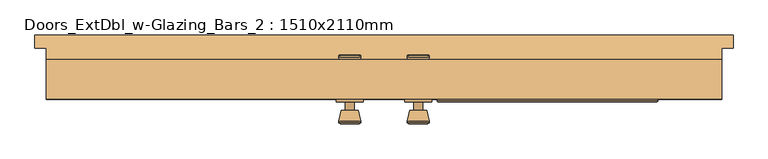
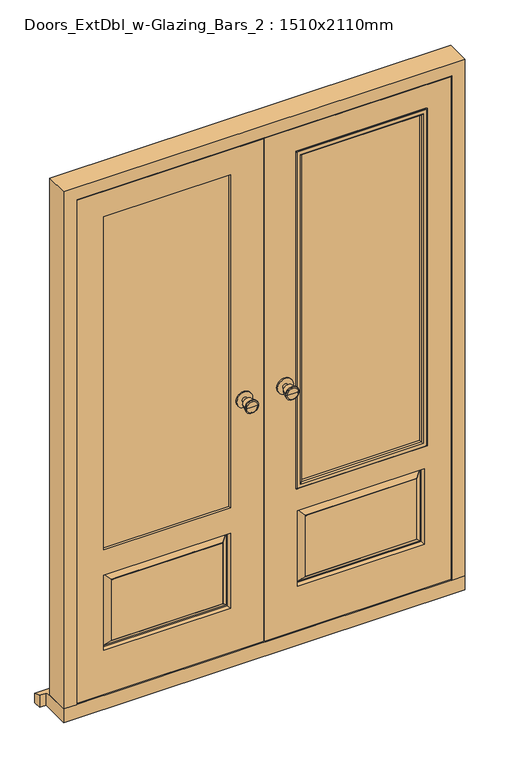
"""IFC4 building model written with IfcOpenShell, lengths in millimetres: door geometry, Doors_ExtDbl_w-Glazing_Bars_2 : 1510x2110mm."""

from ifc_helpers import new_model, si_unit, point, frame, frame_2d, origin, place, context, project, spatial, polyline, circle_curve, ellipse_curve, trimmed, segment, composite_curve, outline, extrude, faceted_brep, source, transform, mapped, element, save
from ifc_brep_helpers import plane_surface, cylinder_surface, revolved_surface, advanced_brep


def doors_extdbl_w_glazing_bars_2_1510x2110mm_e5cd3545(model_context):
    return source(origin(), model_context, "Body", "SolidModel", [
        advanced_brep(
        [(76.5, -18.4, 1050.0), (86.5, -18.4, 1050.0), (66.5, -18.4, 1050.0), (96.9758676, -67.4, 1050.0), (76.5, -67.4, 1050.0), (56.0241324, -67.4, 1050.0), (101.5, -65.5721319, 1050.0), (51.5, -65.5721319, 1050.0), (101.5, -62.1084537, 1050.0), (51.5, -62.1084537, 1050.0), (95.136236, -37.4, 1050.0), (57.863764, -37.4, 1050.0), (86.5, -37.4, 1050.0), (66.5, -37.4, 1050.0)],
        [
            (0, 1),
            (1, 2, circle_curve(frame((76.5, -18.4, 1050.0), z_axis=(0.0, 1.0, 0.0), x_axis=(-1.0, 0.0, 0.0)), 10.0)),
            (2, 0),
            (2, 1, circle_curve(frame((76.5, -18.4, 1050.0), z_axis=(0.0, 1.0, 0.0), x_axis=(-1.0, 0.0, 0.0)), 10.0)),
            (3, 4),
            (4, 5),
            (5, 3, circle_curve(frame((76.5, -67.4, 1050.0), z_axis=(0.0, -1.0, 0.0), x_axis=(-1.0, 0.0, 0.0)), 20.4758676)),
            (3, 5, circle_curve(frame((76.5, -67.4, 1050.0), z_axis=(0.0, -1.0, 0.0), x_axis=(-1.0, 0.0, 0.0)), 20.4758676)),
            (6, 3),
            (5, 7),
            (7, 6, circle_curve(frame((76.5, -65.5721319, 1050.0), z_axis=(0.0, -1.0, 0.0), x_axis=(-1.0, 0.0, 0.0)), 25.0)),
            (6, 7, circle_curve(frame((76.5, -65.5721319, 1050.0), z_axis=(0.0, -1.0, 0.0), x_axis=(-1.0, 0.0, 0.0)), 25.0)),
            (8, 6),
            (7, 9),
            (9, 8, circle_curve(frame((76.5, -62.1084537, 1050.0), z_axis=(0.0, -1.0, 0.0), x_axis=(-1.0, 0.0, 0.0)), 25.0)),
            (8, 9, circle_curve(frame((76.5, -62.1084537, 1050.0), z_axis=(0.0, -1.0, 0.0), x_axis=(-1.0, 0.0, 0.0)), 25.0)),
            (10, 8),
            (9, 11),
            (11, 10, circle_curve(frame((76.5, -37.4, 1050.0), z_axis=(0.0, -1.0, 0.0), x_axis=(-1.0, 0.0, 0.0)), 18.636236)),
            (10, 11, circle_curve(frame((76.5, -37.4, 1050.0), z_axis=(0.0, -1.0, 0.0), x_axis=(-1.0, 0.0, 0.0)), 18.636236)),
            (12, 10),
            (11, 13),
            (13, 12, circle_curve(frame((76.5, -37.4, 1050.0), z_axis=(0.0, -1.0, 0.0), x_axis=(-1.0, 0.0, 0.0)), 10.0)),
            (12, 13, circle_curve(frame((76.5, -37.4, 1050.0), z_axis=(0.0, -1.0, 0.0), x_axis=(-1.0, 0.0, 0.0)), 10.0)),
            (1, 12),
            (13, 2),
        ],
        [
            plane_surface(frame((76.5, -18.4, 1050.0), z_axis=(0.0, 1.0, 0.0), x_axis=(-1.0, 0.0, 0.0))),
            plane_surface(frame((76.5, -67.4, 1050.0), z_axis=(0.0, -1.0, 0.0), x_axis=(-1.0, 0.0, 0.0))),
            revolved_surface(polyline([(56.0241324, -67.4, 1050.0), (51.5, -65.5721319, 1050.0)]), (76.5, -18.4, 1050.0), (0.0, 1.0, 0.0)),
            cylinder_surface(frame((76.5, -18.4, 1050.0), z_axis=(0.0, 1.0, 0.0), x_axis=(-1.0, 0.0, 0.0)), 25.0),
            revolved_surface(polyline([(51.5, -62.1084537, 1050.0), (57.863764, -37.4, 1050.0)]), (76.5, -18.4, 1050.0), (0.0, 1.0, 0.0)),
            plane_surface(frame((76.5, -37.4, 1050.0), z_axis=(0.0, 1.0, 0.0), x_axis=(-1.0, 0.0, 0.0))),
            cylinder_surface(frame((76.5, -18.4, 1050.0), z_axis=(0.0, 1.0, 0.0), x_axis=(-1.0, 0.0, 0.0)), 10.0),
        ],
        [
            (0, [[1, 2, 3]]),
            (0, [[-3, 4, -1]]),
            (1, [[5, 6, 7]]),
            (1, [[-6, -5, 8]]),
            (2, [[9, -7, 10, 11]]),
            (2, [[-10, -8, -9, 12]]),
            (3, [[13, -11, 14, 15]]),
            (3, [[-14, -12, -13, 16]]),
            (4, [[17, -15, 18, 19]]),
            (4, [[-18, -16, -17, 20]]),
            (5, [[21, -19, 22, 23]]),
            (5, [[-22, -20, -21, 24]]),
            (6, [[25, -23, 26, -2]]),
            (6, [[-26, -24, -25, -4]]),
        ],
    ),
        extrude(outline(composite_curve([segment(trimmed(circle_curve(frame_2d((1050.0, 76.5)), 30.0), [point((1050.0, 46.5))], [point((1050.0, 106.5))], False, "CARTESIAN"), True, "CONTINUOUS"), segment(trimmed(circle_curve(frame_2d((1050.0, 76.5)), 30.0), [point((1050.0, 106.5))], [point((1050.0, 46.5))], False, "CARTESIAN"), True, "CONTINUOUS")], self_intersect=False)), frame((0.0, -18.4, 0.0), z_axis=(0.0, 1.0, 0.0), x_axis=(0.0, 0.0, 1.0)), (0.0, 0.0, 1.0), 6.0),
        advanced_brep(
        [(76.5, 37.6, 1050.0), (66.5, 37.6, 1050.0), (86.5, 37.6, 1050.0), (96.9758676, 86.6, 1050.0), (56.0241324, 86.6, 1050.0), (76.5, 86.6, 1050.0), (101.5, 84.7721319, 1050.0), (51.5, 84.7721319, 1050.0), (101.5, 81.3084537, 1050.0), (51.5, 81.3084537, 1050.0), (95.136236, 56.6, 1050.0), (57.863764, 56.6, 1050.0), (86.5, 56.6, 1050.0), (66.5, 56.6, 1050.0)],
        [
            (0, 1),
            (1, 2, circle_curve(frame((76.5, 37.6, 1050.0), z_axis=(0.0, -1.0, 0.0), x_axis=(-1.0, 0.0, 0.0)), 10.0)),
            (2, 0),
            (2, 1, circle_curve(frame((76.5, 37.6, 1050.0), z_axis=(0.0, -1.0, 0.0), x_axis=(-1.0, 0.0, 0.0)), 10.0)),
            (3, 4, circle_curve(frame((76.5, 86.6, 1050.0), z_axis=(0.0, 1.0, 0.0), x_axis=(-1.0, 0.0, 0.0)), 20.4758676)),
            (4, 5),
            (5, 3),
            (4, 3, circle_curve(frame((76.5, 86.6, 1050.0), z_axis=(0.0, 1.0, 0.0), x_axis=(-1.0, 0.0, 0.0)), 20.4758676)),
            (6, 7, circle_curve(frame((76.5, 84.7721319, 1050.0), z_axis=(0.0, 1.0, 0.0), x_axis=(-1.0, 0.0, 0.0)), 25.0)),
            (7, 4),
            (3, 6),
            (7, 6, circle_curve(frame((76.5, 84.7721319, 1050.0), z_axis=(0.0, 1.0, 0.0), x_axis=(-1.0, 0.0, 0.0)), 25.0)),
            (8, 9, circle_curve(frame((76.5, 81.3084537, 1050.0), z_axis=(0.0, 1.0, 0.0), x_axis=(-1.0, 0.0, 0.0)), 25.0)),
            (9, 7),
            (6, 8),
            (9, 8, circle_curve(frame((76.5, 81.3084537, 1050.0), z_axis=(0.0, 1.0, 0.0), x_axis=(-1.0, 0.0, 0.0)), 25.0)),
            (10, 11, circle_curve(frame((76.5, 56.6, 1050.0), z_axis=(0.0, 1.0, 0.0), x_axis=(-1.0, 0.0, 0.0)), 18.636236)),
            (11, 9),
            (8, 10),
            (11, 10, circle_curve(frame((76.5, 56.6, 1050.0), z_axis=(0.0, 1.0, 0.0), x_axis=(-1.0, 0.0, 0.0)), 18.636236)),
            (12, 13, circle_curve(frame((76.5, 56.6, 1050.0), z_axis=(0.0, 1.0, 0.0), x_axis=(-1.0, 0.0, 0.0)), 10.0)),
            (13, 11),
            (10, 12),
            (13, 12, circle_curve(frame((76.5, 56.6, 1050.0), z_axis=(0.0, 1.0, 0.0), x_axis=(-1.0, 0.0, 0.0)), 10.0)),
            (1, 13),
            (12, 2),
        ],
        [
            plane_surface(frame((76.5, 37.6, 1050.0), z_axis=(0.0, -1.0, 0.0), x_axis=(-1.0, 0.0, 0.0))),
            plane_surface(frame((76.5, 86.6, 1050.0), z_axis=(0.0, 1.0, 0.0), x_axis=(-1.0, 0.0, 0.0))),
            revolved_surface(polyline([(56.0241324, 86.6, 1050.0), (51.5, 84.7721319, 1050.0)]), (76.5, 37.6, 1050.0), (0.0, -1.0, 0.0)),
            cylinder_surface(frame((76.5, 37.6, 1050.0), z_axis=(0.0, -1.0, 0.0), x_axis=(-1.0, 0.0, 0.0)), 25.0),
            revolved_surface(polyline([(51.5, 81.3084537, 1050.0), (57.863764, 56.6, 1050.0)]), (76.5, 37.6, 1050.0), (0.0, -1.0, 0.0)),
            plane_surface(frame((76.5, 56.6, 1050.0), z_axis=(0.0, -1.0, 0.0), x_axis=(-1.0, 0.0, 0.0))),
            cylinder_surface(frame((76.5, 37.6, 1050.0), z_axis=(0.0, -1.0, 0.0), x_axis=(-1.0, 0.0, 0.0)), 10.0),
        ],
        [
            (0, [[1, 2, 3]]),
            (0, [[-3, 4, -1]]),
            (1, [[5, 6, 7]]),
            (1, [[8, -7, -6]]),
            (2, [[9, 10, -5, 11]]),
            (2, [[12, -11, -8, -10]]),
            (3, [[13, 14, -9, 15]]),
            (3, [[16, -15, -12, -14]]),
            (4, [[17, 18, -13, 19]]),
            (4, [[20, -19, -16, -18]]),
            (5, [[21, 22, -17, 23]]),
            (5, [[24, -23, -20, -22]]),
            (6, [[-2, 25, -21, 26]]),
            (6, [[-4, -26, -24, -25]]),
        ],
    ),
        extrude(outline(composite_curve([segment(trimmed(circle_curve(frame_2d((1050.0, 76.5)), 30.0), [point((1050.0, 46.5))], [point((1050.0, 106.5))], False, "CARTESIAN"), True, "CONTINUOUS"), segment(trimmed(circle_curve(frame_2d((1050.0, 76.5)), 30.0), [point((1050.0, 106.5))], [point((1050.0, 46.5))], False, "CARTESIAN"), True, "CONTINUOUS")], self_intersect=False)), frame((0.0, 31.6, 0.0), z_axis=(0.0, 1.0, 0.0), x_axis=(0.0, 0.0, 1.0)), (0.0, 0.0, 1.0), 6.0),
        advanced_brep(
        [(-76.5, -18.4, 1050.0), (-66.5, -18.4, 1050.0), (-86.5, -18.4, 1050.0), (-56.0241324, -67.4, 1050.0), (-76.5, -67.4, 1050.0), (-96.9758676, -67.4, 1050.0), (-51.5, -65.5721319, 1050.0), (-101.5, -65.5721319, 1050.0), (-51.5, -62.1084537, 1050.0), (-101.5, -62.1084537, 1050.0), (-57.863764, -37.4, 1050.0), (-95.136236, -37.4, 1050.0), (-66.5, -37.4, 1050.0), (-86.5, -37.4, 1050.0)],
        [
            (0, 1),
            (1, 2, circle_curve(frame((-76.5, -18.4, 1050.0), z_axis=(0.0, 1.0, 0.0), x_axis=(-1.0, 0.0, 0.0)), 10.0)),
            (2, 0),
            (2, 1, circle_curve(frame((-76.5, -18.4, 1050.0), z_axis=(0.0, 1.0, 0.0), x_axis=(-1.0, 0.0, 0.0)), 10.0)),
            (3, 4),
            (4, 5),
            (5, 3, circle_curve(frame((-76.5, -67.4, 1050.0), z_axis=(0.0, -1.0, 0.0), x_axis=(-1.0, 0.0, 0.0)), 20.4758676)),
            (3, 5, circle_curve(frame((-76.5, -67.4, 1050.0), z_axis=(0.0, -1.0, 0.0), x_axis=(-1.0, 0.0, 0.0)), 20.4758676)),
            (6, 3),
            (5, 7),
            (7, 6, circle_curve(frame((-76.5, -65.5721319, 1050.0), z_axis=(0.0, -1.0, 0.0), x_axis=(-1.0, 0.0, 0.0)), 25.0)),
            (6, 7, circle_curve(frame((-76.5, -65.5721319, 1050.0), z_axis=(0.0, -1.0, 0.0), x_axis=(-1.0, 0.0, 0.0)), 25.0)),
            (8, 6),
            (7, 9),
            (9, 8, circle_curve(frame((-76.5, -62.1084537, 1050.0), z_axis=(0.0, -1.0, 0.0), x_axis=(-1.0, 0.0, 0.0)), 25.0)),
            (8, 9, circle_curve(frame((-76.5, -62.1084537, 1050.0), z_axis=(0.0, -1.0, 0.0), x_axis=(-1.0, 0.0, 0.0)), 25.0)),
            (10, 8),
            (9, 11),
            (11, 10, circle_curve(frame((-76.5, -37.4, 1050.0), z_axis=(0.0, -1.0, 0.0), x_axis=(-1.0, 0.0, 0.0)), 18.636236)),
            (10, 11, circle_curve(frame((-76.5, -37.4, 1050.0), z_axis=(0.0, -1.0, 0.0), x_axis=(-1.0, 0.0, 0.0)), 18.636236)),
            (12, 10),
            (11, 13),
            (13, 12, circle_curve(frame((-76.5, -37.4, 1050.0), z_axis=(0.0, -1.0, 0.0), x_axis=(-1.0, 0.0, 0.0)), 10.0)),
            (12, 13, circle_curve(frame((-76.5, -37.4, 1050.0), z_axis=(0.0, -1.0, 0.0), x_axis=(-1.0, 0.0, 0.0)), 10.0)),
            (1, 12),
            (13, 2),
        ],
        [
            plane_surface(frame((-76.5, -18.4, 1050.0), z_axis=(0.0, 1.0, 0.0), x_axis=(-1.0, 0.0, 0.0))),
            plane_surface(frame((-76.5, -67.4, 1050.0), z_axis=(0.0, -1.0, 0.0), x_axis=(-1.0, 0.0, 0.0))),
            revolved_surface(polyline([(-96.9758676, -67.4, 1050.0), (-101.5, -65.5721319, 1050.0)]), (-76.5, -18.4, 1050.0), (0.0, 1.0, 0.0)),
            cylinder_surface(frame((-76.5, -18.4, 1050.0), z_axis=(0.0, 1.0, 0.0), x_axis=(-1.0, 0.0, 0.0)), 25.0),
            revolved_surface(polyline([(-101.5, -62.1084537, 1050.0), (-95.136236, -37.4, 1050.0)]), (-76.5, -18.4, 1050.0), (0.0, 1.0, 0.0)),
            plane_surface(frame((-76.5, -37.4, 1050.0), z_axis=(0.0, 1.0, 0.0), x_axis=(-1.0, 0.0, 0.0))),
            cylinder_surface(frame((-76.5, -18.4, 1050.0), z_axis=(0.0, 1.0, 0.0), x_axis=(-1.0, 0.0, 0.0)), 10.0),
        ],
        [
            (0, [[1, 2, 3]]),
            (0, [[-3, 4, -1]]),
            (1, [[5, 6, 7]]),
            (1, [[-6, -5, 8]]),
            (2, [[9, -7, 10, 11]]),
            (2, [[-10, -8, -9, 12]]),
            (3, [[13, -11, 14, 15]]),
            (3, [[-14, -12, -13, 16]]),
            (4, [[17, -15, 18, 19]]),
            (4, [[-18, -16, -17, 20]]),
            (5, [[21, -19, 22, 23]]),
            (5, [[-22, -20, -21, 24]]),
            (6, [[25, -23, 26, -2]]),
            (6, [[-26, -24, -25, -4]]),
        ],
    ),
        extrude(outline(composite_curve([segment(trimmed(circle_curve(frame_2d((1050.0, -76.5)), 30.0), [point((1050.0, -106.5))], [point((1050.0, -46.5))], False, "CARTESIAN"), True, "CONTINUOUS"), segment(trimmed(circle_curve(frame_2d((1050.0, -76.5)), 30.0), [point((1050.0, -46.5))], [point((1050.0, -106.5))], False, "CARTESIAN"), True, "CONTINUOUS")], self_intersect=False)), frame((0.0, -18.4, 0.0), z_axis=(0.0, 1.0, 0.0), x_axis=(0.0, 0.0, 1.0)), (0.0, 0.0, 1.0), 6.0),
        advanced_brep(
        [(-76.5, 37.6, 1050.0), (-86.5, 37.6, 1050.0), (-66.5, 37.6, 1050.0), (-56.0241324, 86.6, 1050.0), (-96.9758676, 86.6, 1050.0), (-76.5, 86.6, 1050.0), (-51.5, 84.7721319, 1050.0), (-101.5, 84.7721319, 1050.0), (-51.5, 81.3084537, 1050.0), (-101.5, 81.3084537, 1050.0), (-57.863764, 56.6, 1050.0), (-95.136236, 56.6, 1050.0), (-66.5, 56.6, 1050.0), (-86.5, 56.6, 1050.0)],
        [
            (0, 1),
            (1, 2, circle_curve(frame((-76.5, 37.6, 1050.0), z_axis=(0.0, -1.0, 0.0), x_axis=(-1.0, 0.0, 0.0)), 10.0)),
            (2, 0),
            (2, 1, circle_curve(frame((-76.5, 37.6, 1050.0), z_axis=(0.0, -1.0, 0.0), x_axis=(-1.0, 0.0, 0.0)), 10.0)),
            (3, 4, circle_curve(frame((-76.5, 86.6, 1050.0), z_axis=(0.0, 1.0, 0.0), x_axis=(-1.0, 0.0, 0.0)), 20.4758676)),
            (4, 5),
            (5, 3),
            (4, 3, circle_curve(frame((-76.5, 86.6, 1050.0), z_axis=(0.0, 1.0, 0.0), x_axis=(-1.0, 0.0, 0.0)), 20.4758676)),
            (6, 7, circle_curve(frame((-76.5, 84.7721319, 1050.0), z_axis=(0.0, 1.0, 0.0), x_axis=(-1.0, 0.0, 0.0)), 25.0)),
            (7, 4),
            (3, 6),
            (7, 6, circle_curve(frame((-76.5, 84.7721319, 1050.0), z_axis=(0.0, 1.0, 0.0), x_axis=(-1.0, 0.0, 0.0)), 25.0)),
            (8, 9, circle_curve(frame((-76.5, 81.3084537, 1050.0), z_axis=(0.0, 1.0, 0.0), x_axis=(-1.0, 0.0, 0.0)), 25.0)),
            (9, 7),
            (6, 8),
            (9, 8, circle_curve(frame((-76.5, 81.3084537, 1050.0), z_axis=(0.0, 1.0, 0.0), x_axis=(-1.0, 0.0, 0.0)), 25.0)),
            (10, 11, circle_curve(frame((-76.5, 56.6, 1050.0), z_axis=(0.0, 1.0, 0.0), x_axis=(-1.0, 0.0, 0.0)), 18.636236)),
            (11, 9),
            (8, 10),
            (11, 10, circle_curve(frame((-76.5, 56.6, 1050.0), z_axis=(0.0, 1.0, 0.0), x_axis=(-1.0, 0.0, 0.0)), 18.636236)),
            (12, 13, circle_curve(frame((-76.5, 56.6, 1050.0), z_axis=(0.0, 1.0, 0.0), x_axis=(-1.0, 0.0, 0.0)), 10.0)),
            (13, 11),
            (10, 12),
            (13, 12, circle_curve(frame((-76.5, 56.6, 1050.0), z_axis=(0.0, 1.0, 0.0), x_axis=(-1.0, 0.0, 0.0)), 10.0)),
            (1, 13),
            (12, 2),
        ],
        [
            plane_surface(frame((-76.5, 37.6, 1050.0), z_axis=(0.0, -1.0, 0.0), x_axis=(-1.0, 0.0, 0.0))),
            plane_surface(frame((-76.5, 86.6, 1050.0), z_axis=(0.0, 1.0, 0.0), x_axis=(-1.0, 0.0, 0.0))),
            revolved_surface(polyline([(-96.9758676, 86.6, 1050.0), (-101.5, 84.7721319, 1050.0)]), (-76.5, 37.6, 1050.0), (0.0, -1.0, 0.0)),
            cylinder_surface(frame((-76.5, 37.6, 1050.0), z_axis=(0.0, -1.0, 0.0), x_axis=(-1.0, 0.0, 0.0)), 25.0),
            revolved_surface(polyline([(-101.5, 81.3084537, 1050.0), (-95.136236, 56.6, 1050.0)]), (-76.5, 37.6, 1050.0), (0.0, -1.0, 0.0)),
            plane_surface(frame((-76.5, 56.6, 1050.0), z_axis=(0.0, -1.0, 0.0), x_axis=(-1.0, 0.0, 0.0))),
            cylinder_surface(frame((-76.5, 37.6, 1050.0), z_axis=(0.0, -1.0, 0.0), x_axis=(-1.0, 0.0, 0.0)), 10.0),
        ],
        [
            (0, [[1, 2, 3]]),
            (0, [[-3, 4, -1]]),
            (1, [[5, 6, 7]]),
            (1, [[8, -7, -6]]),
            (2, [[9, 10, -5, 11]]),
            (2, [[12, -11, -8, -10]]),
            (3, [[13, 14, -9, 15]]),
            (3, [[16, -15, -12, -14]]),
            (4, [[17, 18, -13, 19]]),
            (4, [[20, -19, -16, -18]]),
            (5, [[21, 22, -17, 23]]),
            (5, [[24, -23, -20, -22]]),
            (6, [[-2, 25, -21, 26]]),
            (6, [[-4, -26, -24, -25]]),
        ],
    ),
        extrude(outline(composite_curve([segment(trimmed(circle_curve(frame_2d((1050.0, -76.5)), 30.0), [point((1050.0, -106.5))], [point((1050.0, -46.5))], False, "CARTESIAN"), True, "CONTINUOUS"), segment(trimmed(circle_curve(frame_2d((1050.0, -76.5)), 30.0), [point((1050.0, -46.5))], [point((1050.0, -106.5))], False, "CARTESIAN"), True, "CONTINUOUS")], self_intersect=False)), frame((0.0, 31.6, 0.0), z_axis=(0.0, 1.0, 0.0), x_axis=(0.0, 0.0, 1.0)), (0.0, 0.0, 1.0), 6.0),
        faceted_brep([(684.5, 76.6, 54.5), (755.0, 76.6, 54.5), (755.0, -12.4, 54.5), (706.5, -12.4, 54.5), (706.5, 34.6, 54.5), (684.5, 34.6, 54.5), (684.5, 76.6, 2039.5), (-684.5, 76.6, 2039.5), (-684.5, 76.6, 54.5), (-755.0, 76.6, 54.5), (-755.0, 76.6, 2110.0), (755.0, 76.6, 2110.0), (755.0, -12.4, 2110.0), (-755.0, -12.4, 2110.0), (-755.0, -12.4, 54.5), (-706.5, -12.4, 54.5), (-706.5, -12.4, 2061.5), (706.5, -12.4, 2061.5), (706.5, 34.6, 2061.5), (-706.5, 34.6, 2061.5), (-706.5, 34.6, 54.5), (-684.5, 34.6, 54.5), (-684.5, 34.6, 2039.5), (684.5, 34.6, 2039.5)], [[[0, 1, 2, 3, 4, 5]], [[1, 0, 6, 7, 8, 9, 10, 11]], [[2, 1, 11, 12]], [[3, 2, 12, 13, 14, 15, 16, 17]], [[4, 3, 17, 18]], [[5, 4, 18, 19, 20, 21, 22, 23]], [[0, 5, 23, 6]], [[8, 7, 22, 21]], [[9, 8, 21, 20, 15, 14]], [[10, 9, 14, 13]], [[16, 15, 20, 19]], [[11, 10, 13, 12]], [[17, 16, 19, 18]], [[7, 6, 23, 22]]]),
        faceted_brep([(703.5, -12.4, 58.5), (703.5, -12.4, 2058.5), (1.5, -12.4, 2058.5), (1.5, -12.4, 58.5), (603.5, -12.4, 1958.5), (603.5, -12.4, 633.5), (126.5, -12.4, 633.5), (126.5, -12.4, 1958.5), (603.5, -12.4, 533.5), (603.5, -12.4, 233.5), (126.5, -12.4, 233.5), (126.5, -12.4, 533.5), (573.5, -12.4, 263.5), (573.5, -12.4, 503.5), (156.5, -12.4, 503.5), (156.5, -12.4, 263.5), (703.5, 31.6, 58.5), (1.5, 31.6, 58.5), (1.5, 31.6, 2058.5), (703.5, 31.6, 2058.5), (603.5, 31.6, 1958.5), (126.5, 31.6, 1958.5), (126.5, 31.6, 633.5), (603.5, 31.6, 633.5), (126.5, 31.6, 533.5), (126.5, 31.6, 233.5), (603.5, 31.6, 233.5), (603.5, 31.6, 533.5), (156.5, 31.6, 263.5), (156.5, 31.6, 503.5), (573.5, 31.6, 503.5), (573.5, 31.6, 263.5), (129.5, 16.6, 530.5), (129.5, 16.6, 236.5), (154.5, 30.6, 505.5), (154.5, 30.6, 261.5), (134.5, 16.6, 241.5), (134.5, 16.6, 525.5), (156.5, 30.6, 263.5), (156.5, 30.6, 503.5), (600.5, 16.6, 236.5), (575.5, 30.6, 261.5), (595.5, 16.6, 241.5), (573.5, 30.6, 263.5), (600.5, 16.6, 530.5), (575.5, 30.6, 505.5), (595.5, 16.6, 525.5), (573.5, 30.6, 503.5), (600.5, 2.6, 530.5), (600.5, 2.6, 236.5), (575.5, -11.4, 505.5), (575.5, -11.4, 261.5), (595.5, 2.6, 241.5), (595.5, 2.6, 525.5), (573.5, -11.4, 263.5), (573.5, -11.4, 503.5), (129.5, 2.6, 236.5), (154.5, -11.4, 261.5), (134.5, 2.6, 241.5), (156.5, -11.4, 263.5), (129.5, 2.6, 530.5), (154.5, -11.4, 505.5), (134.5, 2.6, 525.5), (156.5, -11.4, 503.5)], [[[0, 1, 2, 3], [4, 5, 6, 7], [8, 9, 10, 11]], [[12, 13, 14, 15]], [[16, 17, 18, 19], [20, 21, 22, 23], [24, 25, 26, 27]], [[28, 29, 30, 31]], [[1, 0, 16, 19]], [[2, 1, 19, 18]], [[3, 2, 18, 17]], [[0, 3, 17, 16]], [[5, 4, 20, 23]], [[6, 5, 23, 22]], [[7, 6, 22, 21]], [[4, 7, 21, 20]], [[32, 33, 25, 24]], [[34, 35, 36, 37]], [[28, 38, 39, 29]], [[25, 33, 40, 26]], [[36, 35, 41, 42]], [[38, 28, 31, 43]], [[26, 40, 44, 27]], [[42, 41, 45, 46]], [[43, 31, 30, 47]], [[32, 24, 27, 44]], [[33, 32, 44, 40], [37, 36, 42, 46]], [[34, 37, 46, 45]], [[35, 34, 45, 41], [39, 38, 43, 47]], [[29, 39, 47, 30]], [[48, 49, 9, 8]], [[50, 51, 52, 53]], [[12, 54, 55, 13]], [[9, 49, 56, 10]], [[52, 51, 57, 58]], [[54, 12, 15, 59]], [[10, 56, 60, 11]], [[58, 57, 61, 62]], [[59, 15, 14, 63]], [[48, 8, 11, 60]], [[49, 48, 60, 56], [53, 52, 58, 62]], [[50, 53, 62, 61]], [[51, 50, 61, 57], [55, 54, 59, 63]], [[13, 55, 63, 14]]]),
        faceted_brep([(-703.5, -12.4, 58.5), (-1.5, -12.4, 58.5), (-1.5, -12.4, 2058.5), (-703.5, -12.4, 2058.5), (-126.5, -12.4, 1958.5), (-126.5, -12.4, 633.5), (-603.5, -12.4, 633.5), (-603.5, -12.4, 1958.5), (-126.5, -12.4, 533.5), (-126.5, -12.4, 233.5), (-603.5, -12.4, 233.5), (-603.5, -12.4, 533.5), (-156.5, -12.4, 263.5), (-156.5, -12.4, 503.5), (-573.5, -12.4, 503.5), (-573.5, -12.4, 263.5), (-703.5, 31.6, 58.5), (-703.5, 31.6, 2058.5), (-1.5, 31.6, 2058.5), (-1.5, 31.6, 58.5), (-126.5, 31.6, 1958.5), (-603.5, 31.6, 1958.5), (-603.5, 31.6, 633.5), (-126.5, 31.6, 633.5), (-603.5, 31.6, 533.5), (-603.5, 31.6, 233.5), (-126.5, 31.6, 233.5), (-126.5, 31.6, 533.5), (-573.5, 31.6, 263.5), (-573.5, 31.6, 503.5), (-156.5, 31.6, 503.5), (-156.5, 31.6, 263.5), (-573.5, 30.6, 263.5), (-573.5, 30.6, 503.5), (-595.5, 16.6, 241.5), (-595.5, 16.6, 525.5), (-575.5, 30.6, 505.5), (-575.5, 30.6, 261.5), (-600.5, 16.6, 530.5), (-600.5, 16.6, 236.5), (-156.5, 30.6, 503.5), (-134.5, 16.6, 525.5), (-154.5, 30.6, 505.5), (-129.5, 16.6, 530.5), (-156.5, 30.6, 263.5), (-134.5, 16.6, 241.5), (-154.5, 30.6, 261.5), (-129.5, 16.6, 236.5), (-129.5, 2.6, 530.5), (-129.5, 2.6, 236.5), (-154.5, -11.4, 505.5), (-154.5, -11.4, 261.5), (-134.5, 2.6, 241.5), (-134.5, 2.6, 525.5), (-156.5, -11.4, 263.5), (-156.5, -11.4, 503.5), (-600.5, 2.6, 236.5), (-575.5, -11.4, 261.5), (-595.5, 2.6, 241.5), (-573.5, -11.4, 263.5), (-600.5, 2.6, 530.5), (-575.5, -11.4, 505.5), (-595.5, 2.6, 525.5), (-573.5, -11.4, 503.5)], [[[0, 1, 2, 3], [4, 5, 6, 7], [8, 9, 10, 11]], [[12, 13, 14, 15]], [[16, 17, 18, 19], [20, 21, 22, 23], [24, 25, 26, 27]], [[28, 29, 30, 31]], [[1, 0, 16, 19]], [[2, 1, 19, 18]], [[3, 2, 18, 17]], [[0, 3, 17, 16]], [[5, 4, 20, 23]], [[6, 5, 23, 22]], [[7, 6, 22, 21]], [[4, 7, 21, 20]], [[32, 33, 29, 28]], [[34, 35, 36, 37]], [[24, 38, 39, 25]], [[29, 33, 40, 30]], [[36, 35, 41, 42]], [[38, 24, 27, 43]], [[30, 40, 44, 31]], [[42, 41, 45, 46]], [[43, 27, 26, 47]], [[32, 28, 31, 44]], [[37, 36, 42, 46], [33, 32, 44, 40]], [[34, 37, 46, 45]], [[39, 38, 43, 47], [35, 34, 45, 41]], [[25, 39, 47, 26]], [[48, 49, 9, 8]], [[50, 51, 52, 53]], [[12, 54, 55, 13]], [[9, 49, 56, 10]], [[52, 51, 57, 58]], [[54, 12, 15, 59]], [[10, 56, 60, 11]], [[58, 57, 61, 62]], [[59, 15, 14, 63]], [[48, 8, 11, 60]], [[49, 48, 60, 56], [53, 52, 58, 62]], [[50, 53, 62, 61]], [[51, 50, 61, 57], [55, 54, 59, 63]], [[13, 55, 63, 14]]]),
        faceted_brep([(780.0, 131.6, 0.0), (780.0, 131.6, 38.5947221), (780.0, 101.6, 47.2703282), (780.0, 101.6, 0.0), (-780.0, 131.6, 38.5947221), (-780.0, 131.6, 0.0), (-780.0, 101.6, 0.0), (-780.0, 101.6, 47.2703282), (755.0, 101.6, 0.0), (755.0, -12.4, 0.0), (-755.0, -12.4, 0.0), (-755.0, 101.6, 0.0), (-755.0, 101.6, 47.2703282), (-755.0, 76.6, 54.5), (755.0, 76.6, 54.5), (755.0, 101.6, 47.2703282), (-755.0, -12.4, 54.5), (755.0, -12.4, 54.5)], [[[0, 1, 2, 3]], [[4, 5, 6, 7]], [[5, 0, 3, 8, 9, 10, 11, 6]], [[1, 0, 5, 4]], [[1, 4, 7, 12, 13, 14, 15, 2]], [[13, 16, 17, 14]], [[16, 10, 9, 17]], [[12, 11, 10, 16, 13]], [[11, 12, 7, 6]], [[8, 15, 14, 17, 9]], [[15, 8, 3, 2]]]),
        extrude(outline(polyline([(126.5, 21.6), (603.5, 21.6), (603.5, -2.4), (126.5, -2.4), (126.5, 21.6)])), frame((0.0, 0.0, 633.5), z_axis=(0.0, 0.0, 1.0), x_axis=(1.0, 0.0, 0.0)), (0.0, 0.0, 1.0), 1325.0),
        extrude(outline(polyline([(-603.5, 21.6), (-126.5, 21.6), (-126.5, -2.4), (-603.5, -2.4), (-603.5, 21.6)])), frame((0.0, 0.0, 633.5), z_axis=(0.0, 0.0, 1.0), x_axis=(1.0, 0.0, 0.0)), (0.0, 0.0, 1.0), 1325.0),
        advanced_brep(
        [(118.5, 35.6, 625.5), (118.5, 31.6, 625.5), (118.5, 31.6, 1966.5), (118.5, 35.6, 1966.5), (120.5, 37.6, 627.5), (120.5, 37.6, 1964.5), (138.5, 32.6, 645.5), (133.5, 37.6, 640.5), (133.5, 37.6, 1951.5), (138.5, 32.6, 1946.5), (138.5, 21.6, 645.5), (138.5, 21.6, 1946.5), (126.5, 31.6, 633.5), (126.5, 21.6, 633.5), (126.5, 21.6, 1958.5), (126.5, 31.6, 1958.5), (611.5, 31.6, 1966.5), (611.5, 35.6, 1966.5), (609.5, 37.6, 1964.5), (596.5, 37.6, 1951.5), (591.5, 32.6, 1946.5), (591.5, 21.6, 1946.5), (603.5, 21.6, 1958.5), (603.5, 31.6, 1958.5), (611.5, 31.6, 625.5), (611.5, 35.6, 625.5), (609.5, 37.6, 627.5), (596.5, 37.6, 640.5), (591.5, 32.6, 645.5), (591.5, 21.6, 645.5), (603.5, 21.6, 633.5), (603.5, 31.6, 633.5)],
        [
            (0, 1),
            (1, 2),
            (2, 3),
            (3, 0),
            (4, 0, ellipse_curve(frame((120.5, 35.6, 627.5), z_axis=(-0.7071067811865476, 0.0, 0.7071067811865475), x_axis=(-0.7071067811865475, 0.0, -0.7071067811865476)), 2.8284271, 2.0)),
            (3, 5, ellipse_curve(frame((120.5, 35.6, 1964.5), z_axis=(-0.7071067811865475, 0.0, -0.7071067811865476), x_axis=(0.7071067811865476, 0.0, -0.7071067811865475)), 2.8284271, 2.0)),
            (5, 4),
            (6, 7, ellipse_curve(frame((133.5, 32.6, 640.5), z_axis=(-0.7071067811865476, 0.0, 0.7071067811865475), x_axis=(-0.7071067811865475, 0.0, -0.7071067811865476)), 7.0710678, 5.0)),
            (7, 8),
            (8, 9, ellipse_curve(frame((133.5, 32.6, 1951.5), z_axis=(-0.7071067811865475, 0.0, -0.7071067811865476), x_axis=(0.7071067811865476, 0.0, -0.7071067811865475)), 7.0710678, 5.0)),
            (9, 6),
            (10, 6),
            (9, 11),
            (11, 10),
            (12, 13),
            (13, 14),
            (14, 15),
            (15, 12),
            (2, 16),
            (16, 17),
            (17, 3),
            (17, 18, ellipse_curve(frame((609.5, 35.6, 1964.5), z_axis=(-0.7071067811865476, 0.0, 0.7071067811865474), x_axis=(-0.7071067811865475, 0.0, -0.7071067811865475)), 2.8284271, 2.0)),
            (18, 5),
            (8, 19),
            (19, 20, ellipse_curve(frame((596.5, 32.6, 1951.5), z_axis=(-0.7071067811865476, 0.0, 0.7071067811865474), x_axis=(-0.7071067811865475, 0.0, -0.7071067811865475)), 7.0710678, 5.0)),
            (20, 9),
            (20, 21),
            (21, 11),
            (14, 22),
            (22, 23),
            (23, 15),
            (16, 24),
            (24, 25),
            (25, 17),
            (25, 26, ellipse_curve(frame((609.5, 35.6, 627.5), z_axis=(0.7071067811865474, 0.0, 0.7071067811865476), x_axis=(-0.7071067811865475, 0.0, 0.7071067811865475)), 2.8284271, 2.0)),
            (26, 18),
            (19, 27),
            (27, 28, ellipse_curve(frame((596.5, 32.6, 640.5), z_axis=(0.7071067811865474, 0.0, 0.7071067811865476), x_axis=(-0.7071067811865475, 0.0, 0.7071067811865475)), 7.0710678, 5.0)),
            (28, 20),
            (28, 29),
            (29, 21),
            (22, 30),
            (30, 31),
            (31, 23),
            (24, 1),
            (0, 25),
            (4, 26),
            (7, 27),
            (6, 28),
            (10, 29),
            (13, 30),
            (12, 31),
        ],
        [
            plane_surface(frame((118.5, 31.6, 625.5), z_axis=(-1.0, 0.0, 0.0), x_axis=(0.0, 0.0, 1.0))),
            cylinder_surface(frame((120.5, 35.6, 633.5), z_axis=(0.0, 0.0, -1.0), x_axis=(-1.0, 0.0, 0.0)), 2.0),
            cylinder_surface(frame((133.5, 32.6, 633.5), z_axis=(0.0, 0.0, -1.0), x_axis=(-1.0, 0.0, 0.0)), 5.0),
            plane_surface(frame((138.5, 32.6, 645.5), z_axis=(1.0, 0.0, 0.0), x_axis=(0.0, 0.0, 1.0))),
            plane_surface(frame((126.5, 21.6, 633.5), z_axis=(-1.0, 0.0, 0.0), x_axis=(0.0, 0.0, 1.0))),
            plane_surface(frame((118.5, 31.6, 1966.5), z_axis=(0.0, 0.0, 1.0), x_axis=(1.0, 0.0, 0.0))),
            cylinder_surface(frame((126.5, 35.6, 1964.5), z_axis=(-1.0, 0.0, 0.0), x_axis=(0.0, 0.0, 1.0)), 2.0),
            cylinder_surface(frame((126.5, 32.6, 1951.5), z_axis=(-1.0, 0.0, 0.0), x_axis=(0.0, 0.0, 1.0)), 5.0),
            plane_surface(frame((138.5, 32.6, 1946.5), z_axis=(0.0, 0.0, -1.0), x_axis=(1.0, 0.0, 0.0))),
            plane_surface(frame((126.5, 21.6, 1958.5), z_axis=(0.0, 0.0, 1.0), x_axis=(1.0, 0.0, 0.0))),
            plane_surface(frame((611.5, 31.6, 1966.5), z_axis=(1.0, 0.0, 0.0), x_axis=(0.0, 0.0, -1.0))),
            cylinder_surface(frame((609.5, 35.6, 1958.5), z_axis=(0.0, 0.0, 1.0), x_axis=(1.0, 0.0, 0.0)), 2.0),
            cylinder_surface(frame((596.5, 32.6, 1958.5), z_axis=(0.0, 0.0, 1.0), x_axis=(1.0, 0.0, 0.0)), 5.0),
            plane_surface(frame((591.5, 32.6, 1946.5), z_axis=(-1.0, 0.0, 0.0), x_axis=(0.0, 0.0, -1.0))),
            plane_surface(frame((603.5, 21.6, 1958.5), z_axis=(1.0, 0.0, 0.0), x_axis=(0.0, 0.0, -1.0))),
            plane_surface(frame((611.5, 31.6, 625.5), z_axis=(0.0, 0.0, -1.0), x_axis=(-1.0, 0.0, 0.0))),
            cylinder_surface(frame((603.5, 35.6, 627.5), z_axis=(1.0, 0.0, 0.0), x_axis=(0.0, 0.0, -1.0)), 2.0),
            plane_surface(frame((609.5, 37.6, 627.5), z_axis=(0.0, 1.0, 0.0), x_axis=(-1.0, 0.0, 0.0))),
            cylinder_surface(frame((603.5, 32.6, 640.5), z_axis=(1.0, 0.0, 0.0), x_axis=(0.0, 0.0, -1.0)), 5.0),
            plane_surface(frame((591.5, 32.6, 645.5), z_axis=(0.0, 0.0, 1.0), x_axis=(-1.0, 0.0, 0.0))),
            plane_surface(frame((591.5, 21.6, 645.5), z_axis=(0.0, -1.0, 0.0), x_axis=(-1.0, 0.0, 0.0))),
            plane_surface(frame((603.5, 21.6, 633.5), z_axis=(0.0, 0.0, -1.0), x_axis=(-1.0, 0.0, 0.0))),
            plane_surface(frame((603.5, 31.6, 633.5), z_axis=(0.0, -1.0, 0.0), x_axis=(-1.0, 0.0, 0.0))),
        ],
        [
            (0, [[1, 2, 3, 4]]),
            (1, [[5, -4, 6, 7]]),
            (2, [[8, 9, 10, 11]]),
            (3, [[12, -11, 13, 14]]),
            (4, [[15, 16, 17, 18]]),
            (5, [[-3, 19, 20, 21]]),
            (6, [[-6, -21, 22, 23]]),
            (7, [[-10, 24, 25, 26]]),
            (8, [[-13, -26, 27, 28]]),
            (9, [[-17, 29, 30, 31]]),
            (10, [[-20, 32, 33, 34]]),
            (11, [[-22, -34, 35, 36]]),
            (12, [[-25, 37, 38, 39]]),
            (13, [[-27, -39, 40, 41]]),
            (14, [[-30, 42, 43, 44]]),
            (15, [[-33, 45, -1, 46]]),
            (16, [[-35, -46, -5, 47]]),
            (17, [[-23, -36, -47, -7], [48, -37, -24, -9]]),
            (18, [[-38, -48, -8, 49]]),
            (19, [[-40, -49, -12, 50]]),
            (20, [[51, -42, -29, -16], [-28, -41, -50, -14]]),
            (21, [[-43, -51, -15, 52]]),
            (22, [[-45, -32, -19, -2], [-31, -44, -52, -18]]),
        ],
    ),
        advanced_brep(
        [(603.5, -2.4, 1958.5), (603.5, -12.4, 1958.5), (603.5, -12.4, 633.5), (603.5, -2.4, 633.5), (591.5, -13.4, 1946.5), (591.5, -2.4, 1946.5), (591.5, -2.4, 645.5), (591.5, -13.4, 645.5), (596.5, -18.4, 1951.5), (596.5, -18.4, 640.5), (611.5, -16.4, 1966.5), (609.5, -18.4, 1964.5), (609.5, -18.4, 627.5), (611.5, -16.4, 625.5), (611.5, -12.4, 1966.5), (611.5, -12.4, 625.5), (126.5, -12.4, 633.5), (126.5, -2.4, 633.5), (138.5, -2.4, 645.5), (138.5, -13.4, 645.5), (133.5, -18.4, 640.5), (120.5, -18.4, 627.5), (118.5, -16.4, 625.5), (118.5, -12.4, 625.5), (126.5, -12.4, 1958.5), (126.5, -2.4, 1958.5), (138.5, -2.4, 1946.5), (138.5, -13.4, 1946.5), (133.5, -18.4, 1951.5), (120.5, -18.4, 1964.5), (118.5, -16.4, 1966.5), (118.5, -12.4, 1966.5)],
        [
            (0, 1),
            (1, 2),
            (2, 3),
            (3, 0),
            (4, 5),
            (5, 6),
            (6, 7),
            (7, 4),
            (8, 4, ellipse_curve(frame((596.5, -13.4, 1951.5), z_axis=(0.707106781186552, 0.0, -0.707106781186543), x_axis=(0.7071067811865429, 0.0, 0.707106781186552)), 7.0710678, 5.0)),
            (7, 9, ellipse_curve(frame((596.5, -13.4, 640.5), z_axis=(0.7071067811865431, 0.0, 0.707106781186552), x_axis=(-0.7071067811865521, 0.0, 0.7071067811865429)), 7.0710678, 5.0)),
            (9, 8),
            (10, 11, ellipse_curve(frame((609.5, -16.4, 1964.5), z_axis=(0.707106781186552, 0.0, -0.707106781186543), x_axis=(0.7071067811865429, 0.0, 0.707106781186552)), 2.8284271, 2.0)),
            (11, 12),
            (12, 13, ellipse_curve(frame((609.5, -16.4, 627.5), z_axis=(0.7071067811865431, 0.0, 0.707106781186552), x_axis=(-0.7071067811865521, 0.0, 0.7071067811865429)), 2.8284271, 2.0)),
            (13, 10),
            (14, 10),
            (13, 15),
            (15, 14),
            (2, 16),
            (16, 17),
            (17, 3),
            (6, 18),
            (18, 19),
            (19, 7),
            (19, 20, ellipse_curve(frame((133.5, -13.4, 640.5), z_axis=(0.707106781186552, 0.0, -0.707106781186543), x_axis=(0.7071067811865431, 0.0, 0.7071067811865519)), 7.0710678, 5.0)),
            (20, 9),
            (12, 21),
            (21, 22, ellipse_curve(frame((120.5, -16.4, 627.5), z_axis=(0.707106781186552, 0.0, -0.707106781186543), x_axis=(0.7071067811865431, 0.0, 0.7071067811865519)), 2.8284271, 2.0)),
            (22, 13),
            (22, 23),
            (23, 15),
            (16, 24),
            (24, 25),
            (25, 17),
            (18, 26),
            (26, 27),
            (27, 19),
            (27, 28, ellipse_curve(frame((133.5, -13.4, 1951.5), z_axis=(-0.7071067811865431, 0.0, -0.707106781186552), x_axis=(0.707106781186552, 0.0, -0.707106781186543)), 7.0710678, 5.0)),
            (28, 20),
            (21, 29),
            (29, 30, ellipse_curve(frame((120.5, -16.4, 1964.5), z_axis=(-0.7071067811865431, 0.0, -0.707106781186552), x_axis=(0.707106781186552, 0.0, -0.707106781186543)), 2.8284271, 2.0)),
            (30, 22),
            (30, 31),
            (31, 23),
            (31, 14),
            (1, 24),
            (0, 25),
            (5, 26),
            (4, 27),
            (8, 28),
            (11, 29),
            (10, 30),
        ],
        [
            plane_surface(frame((603.5, -12.4, 1958.5), z_axis=(1.0, 0.0, 0.0), x_axis=(0.0, 0.0, -1.0))),
            plane_surface(frame((591.5, -2.4, 1946.5), z_axis=(-1.0, 0.0, 0.0), x_axis=(0.0, 0.0, -1.0))),
            cylinder_surface(frame((596.5, -13.4, 1958.5), z_axis=(0.0, 0.0, 1.0), x_axis=(1.0, 0.0, 0.0)), 5.0),
            cylinder_surface(frame((609.5, -16.4, 1958.5), z_axis=(0.0, 0.0, 1.0), x_axis=(1.0, 0.0, 0.0)), 2.0),
            plane_surface(frame((611.5, -16.4, 1966.5), z_axis=(1.0, 0.0, 0.0), x_axis=(0.0, 0.0, -1.0))),
            plane_surface(frame((603.5, -12.4, 633.5), z_axis=(0.0, 0.0, -1.0), x_axis=(-1.0, 0.0, 0.0))),
            plane_surface(frame((591.5, -2.4, 645.5), z_axis=(0.0, 0.0, 1.0), x_axis=(-1.0, 0.0, 0.0))),
            cylinder_surface(frame((603.5, -13.4, 640.5), z_axis=(1.0, 0.0, 0.0), x_axis=(0.0, 0.0, -1.0)), 5.0),
            cylinder_surface(frame((603.5, -16.4, 627.5), z_axis=(1.0, 0.0, 0.0), x_axis=(0.0, 0.0, -1.0)), 2.0),
            plane_surface(frame((611.5, -16.4, 625.5), z_axis=(0.0, 0.0, -1.0), x_axis=(-1.0, 0.0, 0.0))),
            plane_surface(frame((126.5, -12.4, 633.5), z_axis=(-1.0, 0.0, 0.0), x_axis=(0.0, 0.0, 1.0))),
            plane_surface(frame((138.5, -2.4, 645.5), z_axis=(1.0, 0.0, 0.0), x_axis=(0.0, 0.0, 1.0))),
            cylinder_surface(frame((133.5, -13.4, 633.5), z_axis=(0.0, 0.0, -1.0), x_axis=(-1.0, 0.0, 0.0)), 5.0),
            cylinder_surface(frame((120.5, -16.4, 633.5), z_axis=(0.0, 0.0, -1.0), x_axis=(-1.0, 0.0, 0.0)), 2.0),
            plane_surface(frame((118.5, -16.4, 625.5), z_axis=(-1.0, 0.0, 0.0), x_axis=(0.0, 0.0, 1.0))),
            plane_surface(frame((118.5, -12.4, 1966.5), z_axis=(0.0, 1.0, 0.0), x_axis=(1.0, 0.0, 0.0))),
            plane_surface(frame((126.5, -12.4, 1958.5), z_axis=(0.0, 0.0, 1.0), x_axis=(1.0, 0.0, 0.0))),
            plane_surface(frame((126.5, -2.4, 1958.5), z_axis=(0.0, 1.0, 0.0), x_axis=(1.0, 0.0, 0.0))),
            plane_surface(frame((138.5, -2.4, 1946.5), z_axis=(0.0, 0.0, -1.0), x_axis=(1.0, 0.0, 0.0))),
            cylinder_surface(frame((126.5, -13.4, 1951.5), z_axis=(-1.0, 0.0, 0.0), x_axis=(0.0, 0.0, 1.0)), 5.0),
            plane_surface(frame((133.5, -18.4, 1951.5), z_axis=(0.0, -1.0, 0.0), x_axis=(1.0, 0.0, 0.0))),
            cylinder_surface(frame((126.5, -16.4, 1964.5), z_axis=(-1.0, 0.0, 0.0), x_axis=(0.0, 0.0, 1.0)), 2.0),
            plane_surface(frame((118.5, -16.4, 1966.5), z_axis=(0.0, 0.0, 1.0), x_axis=(1.0, 0.0, 0.0))),
        ],
        [
            (0, [[1, 2, 3, 4]]),
            (1, [[5, 6, 7, 8]]),
            (2, [[9, -8, 10, 11]]),
            (3, [[12, 13, 14, 15]]),
            (4, [[16, -15, 17, 18]]),
            (5, [[-3, 19, 20, 21]]),
            (6, [[-7, 22, 23, 24]]),
            (7, [[-10, -24, 25, 26]]),
            (8, [[-14, 27, 28, 29]]),
            (9, [[-17, -29, 30, 31]]),
            (10, [[-20, 32, 33, 34]]),
            (11, [[-23, 35, 36, 37]]),
            (12, [[-25, -37, 38, 39]]),
            (13, [[-28, 40, 41, 42]]),
            (14, [[-30, -42, 43, 44]]),
            (15, [[-31, -44, 45, -18], [46, -32, -19, -2]]),
            (16, [[-33, -46, -1, 47]]),
            (17, [[-21, -34, -47, -4], [48, -35, -22, -6]]),
            (18, [[-36, -48, -5, 49]]),
            (19, [[-38, -49, -9, 50]]),
            (20, [[51, -40, -27, -13], [-26, -39, -50, -11]]),
            (21, [[-41, -51, -12, 52]]),
            (22, [[-43, -52, -16, -45]]),
        ],
    ),
        advanced_brep(
        [(-611.5, 35.6, 625.5), (-611.5, 31.6, 625.5), (-611.5, 31.6, 1966.5), (-611.5, 35.6, 1966.5), (-609.5, 37.6, 627.5), (-609.5, 37.6, 1964.5), (-591.5, 32.6, 645.5), (-596.5, 37.6, 640.5), (-596.5, 37.6, 1951.5), (-591.5, 32.6, 1946.5), (-591.5, 21.6, 645.5), (-591.5, 21.6, 1946.5), (-603.5, 31.6, 633.5), (-603.5, 21.6, 633.5), (-603.5, 21.6, 1958.5), (-603.5, 31.6, 1958.5), (-118.5, 31.6, 1966.5), (-118.5, 35.6, 1966.5), (-120.5, 37.6, 1964.5), (-133.5, 37.6, 1951.5), (-138.5, 32.6, 1946.5), (-138.5, 21.6, 1946.5), (-126.5, 21.6, 1958.5), (-126.5, 31.6, 1958.5), (-118.5, 31.6, 625.5), (-118.5, 35.6, 625.5), (-120.5, 37.6, 627.5), (-133.5, 37.6, 640.5), (-138.5, 32.6, 645.5), (-138.5, 21.6, 645.5), (-126.5, 21.6, 633.5), (-126.5, 31.6, 633.5)],
        [
            (0, 1),
            (1, 2),
            (2, 3),
            (3, 0),
            (4, 0, ellipse_curve(frame((-609.5, 35.6, 627.5), z_axis=(-0.7071067811865476, 0.0, 0.7071067811865475), x_axis=(-0.7071067811865475, 0.0, -0.7071067811865475)), 2.8284271, 2.0)),
            (3, 5, ellipse_curve(frame((-609.5, 35.6, 1964.5), z_axis=(-0.7071067811865475, 0.0, -0.7071067811865476), x_axis=(0.7071067811865475, 0.0, -0.7071067811865475)), 2.8284271, 2.0)),
            (5, 4),
            (6, 7, ellipse_curve(frame((-596.5, 32.6, 640.5), z_axis=(-0.7071067811865476, 0.0, 0.7071067811865475), x_axis=(-0.7071067811865475, 0.0, -0.7071067811865475)), 7.0710678, 5.0)),
            (7, 8),
            (8, 9, ellipse_curve(frame((-596.5, 32.6, 1951.5), z_axis=(-0.7071067811865475, 0.0, -0.7071067811865476), x_axis=(0.7071067811865475, 0.0, -0.7071067811865475)), 7.0710678, 5.0)),
            (9, 6),
            (10, 6),
            (9, 11),
            (11, 10),
            (12, 13),
            (13, 14),
            (14, 15),
            (15, 12),
            (2, 16),
            (16, 17),
            (17, 3),
            (17, 18, ellipse_curve(frame((-120.5, 35.6, 1964.5), z_axis=(-0.7071067811865475, 0.0, 0.7071067811865475), x_axis=(-0.7071067811865477, 0.0, -0.7071067811865472)), 2.8284271, 2.0)),
            (18, 5),
            (8, 19),
            (19, 20, ellipse_curve(frame((-133.5, 32.6, 1951.5), z_axis=(-0.7071067811865475, 0.0, 0.7071067811865475), x_axis=(-0.7071067811865477, 0.0, -0.7071067811865472)), 7.0710678, 5.0)),
            (20, 9),
            (20, 21),
            (21, 11),
            (14, 22),
            (22, 23),
            (23, 15),
            (16, 24),
            (24, 25),
            (25, 17),
            (25, 26, ellipse_curve(frame((-120.5, 35.6, 627.5), z_axis=(0.7071067811865476, 0.0, 0.7071067811865475), x_axis=(-0.7071067811865475, 0.0, 0.7071067811865475)), 2.8284271, 2.0)),
            (26, 18),
            (19, 27),
            (27, 28, ellipse_curve(frame((-133.5, 32.6, 640.5), z_axis=(0.7071067811865476, 0.0, 0.7071067811865475), x_axis=(-0.7071067811865475, 0.0, 0.7071067811865475)), 7.0710678, 5.0)),
            (28, 20),
            (28, 29),
            (29, 21),
            (22, 30),
            (30, 31),
            (31, 23),
            (24, 1),
            (0, 25),
            (4, 26),
            (7, 27),
            (6, 28),
            (10, 29),
            (13, 30),
            (12, 31),
        ],
        [
            plane_surface(frame((-611.5, 31.6, 625.5), z_axis=(-1.0, 0.0, 0.0), x_axis=(0.0, 0.0, 1.0))),
            cylinder_surface(frame((-609.5, 35.6, 633.5), z_axis=(0.0, 0.0, -1.0), x_axis=(-1.0, 0.0, 0.0)), 2.0),
            cylinder_surface(frame((-596.5, 32.6, 633.5), z_axis=(0.0, 0.0, -1.0), x_axis=(-1.0, 0.0, 0.0)), 5.0),
            plane_surface(frame((-591.5, 32.6, 645.5), z_axis=(1.0, 0.0, 0.0), x_axis=(0.0, 0.0, 1.0))),
            plane_surface(frame((-603.5, 21.6, 633.5), z_axis=(-1.0, 0.0, 0.0), x_axis=(0.0, 0.0, 1.0))),
            plane_surface(frame((-611.5, 31.6, 1966.5), z_axis=(0.0, 0.0, 1.0), x_axis=(1.0, 0.0, 0.0))),
            cylinder_surface(frame((-603.5, 35.6, 1964.5), z_axis=(-1.0, 0.0, 0.0), x_axis=(0.0, 0.0, 1.0)), 2.0),
            cylinder_surface(frame((-603.5, 32.6, 1951.5), z_axis=(-1.0, 0.0, 0.0), x_axis=(0.0, 0.0, 1.0)), 5.0),
            plane_surface(frame((-591.5, 32.6, 1946.5), z_axis=(0.0, 0.0, -1.0), x_axis=(1.0, 0.0, 0.0))),
            plane_surface(frame((-603.5, 21.6, 1958.5), z_axis=(0.0, 0.0, 1.0), x_axis=(1.0, 0.0, 0.0))),
            plane_surface(frame((-118.5, 31.6, 1966.5), z_axis=(1.0, 0.0, 0.0), x_axis=(0.0, 0.0, -1.0))),
            cylinder_surface(frame((-120.5, 35.6, 1958.5), z_axis=(0.0, 0.0, 1.0), x_axis=(1.0, 0.0, 0.0)), 2.0),
            cylinder_surface(frame((-133.5, 32.6, 1958.5), z_axis=(0.0, 0.0, 1.0), x_axis=(1.0, 0.0, 0.0)), 5.0),
            plane_surface(frame((-138.5, 32.6, 1946.5), z_axis=(-1.0, 0.0, 0.0), x_axis=(0.0, 0.0, -1.0))),
            plane_surface(frame((-126.5, 21.6, 1958.5), z_axis=(1.0, 0.0, 0.0), x_axis=(0.0, 0.0, -1.0))),
            plane_surface(frame((-118.5, 31.6, 625.5), z_axis=(0.0, 0.0, -1.0), x_axis=(-1.0, 0.0, 0.0))),
            cylinder_surface(frame((-126.5, 35.6, 627.5), z_axis=(1.0, 0.0, 0.0), x_axis=(0.0, 0.0, -1.0)), 2.0),
            plane_surface(frame((-120.5, 37.6, 627.5), z_axis=(0.0, 1.0, 0.0), x_axis=(-1.0, 0.0, 0.0))),
            cylinder_surface(frame((-126.5, 32.6, 640.5), z_axis=(1.0, 0.0, 0.0), x_axis=(0.0, 0.0, -1.0)), 5.0),
            plane_surface(frame((-138.5, 32.6, 645.5), z_axis=(0.0, 0.0, 1.0), x_axis=(-1.0, 0.0, 0.0))),
            plane_surface(frame((-138.5, 21.6, 645.5), z_axis=(0.0, -1.0, 0.0), x_axis=(-1.0, 0.0, 0.0))),
            plane_surface(frame((-126.5, 21.6, 633.5), z_axis=(0.0, 0.0, -1.0), x_axis=(-1.0, 0.0, 0.0))),
            plane_surface(frame((-126.5, 31.6, 633.5), z_axis=(0.0, -1.0, 0.0), x_axis=(-1.0, 0.0, 0.0))),
        ],
        [
            (0, [[1, 2, 3, 4]]),
            (1, [[5, -4, 6, 7]]),
            (2, [[8, 9, 10, 11]]),
            (3, [[12, -11, 13, 14]]),
            (4, [[15, 16, 17, 18]]),
            (5, [[-3, 19, 20, 21]]),
            (6, [[-6, -21, 22, 23]]),
            (7, [[-10, 24, 25, 26]]),
            (8, [[-13, -26, 27, 28]]),
            (9, [[-17, 29, 30, 31]]),
            (10, [[-20, 32, 33, 34]]),
            (11, [[-22, -34, 35, 36]]),
            (12, [[-25, 37, 38, 39]]),
            (13, [[-27, -39, 40, 41]]),
            (14, [[-30, 42, 43, 44]]),
            (15, [[-33, 45, -1, 46]]),
            (16, [[-35, -46, -5, 47]]),
            (17, [[-23, -36, -47, -7], [48, -37, -24, -9]]),
            (18, [[-38, -48, -8, 49]]),
            (19, [[-40, -49, -12, 50]]),
            (20, [[51, -42, -29, -16], [-28, -41, -50, -14]]),
            (21, [[-43, -51, -15, 52]]),
            (22, [[-45, -32, -19, -2], [-31, -44, -52, -18]]),
        ],
    ),
    ])


if __name__ == "__main__":
    model = new_model("IFC4")
    model_context = context("Model", 3, world=origin())
    ifc_project = project(units=[si_unit("LENGTHUNIT", "METRE", prefix="MILLI")], contexts=[model_context])
    site = spatial("IfcSite", under=ifc_project)
    building = spatial("IfcBuilding", under=site)
    placement = place(None, origin())
    doors_extdbl_w_glazing_bars_2_1510x2110mm_shape = doors_extdbl_w_glazing_bars_2_1510x2110mm_e5cd3545(model_context)
    element("IfcDoor", 1, ObjectType="Doors_ExtDbl_w-Glazing_Bars_2 : 1510x2110mm", at=placement, inside=building, context=model_context, shape_type="MappedRepresentation", body=[
        mapped(doors_extdbl_w_glazing_bars_2_1510x2110mm_shape, transform((0.0, 0.0, 0.0), x_axis=(1.0, 0.0, 0.0), y_axis=(0.0, 1.0, 0.0), z_axis=(0.0, 0.0, 1.0))),
    ])
    save(model, "model.ifc")

# Revit data of these elements
# Type "Doors_ExtDbl_w-Glazing_Bars_2 : 1510x2110mm"
#   Type Mark = "15"
#   Type Comments = "External Double"
#   Operation = "DoubleDoorSingleSwing"
#   Construction Type Id = "GSP4R"
#   Keynote = "L20"
#   Analytic Construction = "1/8 in Pilkington single glazing"
#   Wrap Layers (Int) from Ext = 0' - 6.98819"
#   Wrap Layers (Ext) from Ext = 0' - 4.03543"
#   Visual Light Transmittance = 0.9
#   Top of Intermediate Rail = 1' - 10.6378"
#   Thickness = 0' - 1.73228"
#   Stile Shutting = 0' - 4.92126"
#   Stile - Top Rail = 0' - 3.93701"
#   Stile - Lock Rail = 0' - 3.93701"
#   Stile - Hanging = 0' - 3.93701"
#   Stile - Bottom Rail = 0' - 6.88976"
#   Solar Heat Gain Coefficient = 0.78
#   Rough Width = 4' - 11.44882"
#   Rough Height = 6' - 11.07087"
#   O/A Frame Width = 0' - 2.51969"
#   Heat Transfer Coefficient (U) = 0.6496 BTU/(h·ft²·°F)
#   Handle Z Distance = 3' - 5.33858"
#   Glazing Thickness = 0' - 0.94488"
#   Glazing Bar Thickness = 0' - 0.7874"
#   FrameWidth = 0' - 1.65354"
#   FrameOffset - External = 0' - 0.98425"
#   FrameDepth = 0' - 3.50394"
#   Door Panel Width = 2' - 3.6378"
#   Door Panel Thickness = 0' - 1.73228"
#   Door Panel Height = 6' - 6.74016"
#   Cill Thickness = 0' - 2.14567"
#   Cill Projection = 0' - 1.1811"
#   Handle X Distance = 0' - 2.95276"
#   Height = 6' - 11.07087"
#   Structural Tolerance = 0' - 0.25591"
#   Tolerance = 0' - 0.11811"
#   Undercut = 0' - 0.15748"
#   Width = 4' - 11.44882"
#   Cill Extension = 0' - 0.98425"
#   Cavity Closer Width = 0' - 1.9685"
#   Cavity Closer Offset from Ext = 0' - 4.03543"
#   Cavity Closer Depth = 0' - 3.34646"
#   Vis - Ironmongery = yes
#   Vis - Glazing Bars = yes
#   Vis - Cavity Closers = yes
#   Define Thermal Properties by = 1
#   Function = 1
#   Material Glazing Bars = Door - Panel
#   Material Glass = Door - Glazing
#   Material Door = Door - Panel
#   Material Frame = Door - Frame/Mullion
#   Material Ironmongery = Door - Handle
#   Wall Closure = (empty or 0)
#   Assembly Code = ""
# Element 1 (IfcDoor, "Doors_ExtDbl_w-Glazing_Bars_2 : 1510x2110mm")
#   Materials on its faces: "Door - Panel", "Door - Handle", "Door - Frame/Mullion", "Door - Glazing"
# Materials
#   "Door - Panel": class "Wood", colour RGB 210 159 95, transparency 0, Cost = 0
#   "Door - Glazing": colour RGB 0 0 255, transparency 0.75
#   "Door - Frame/Mullion": class "Wood", colour RGB 212 179 113, transparency 0
#   "Door - Handle": colour RGB 247 247 247, transparency 0
